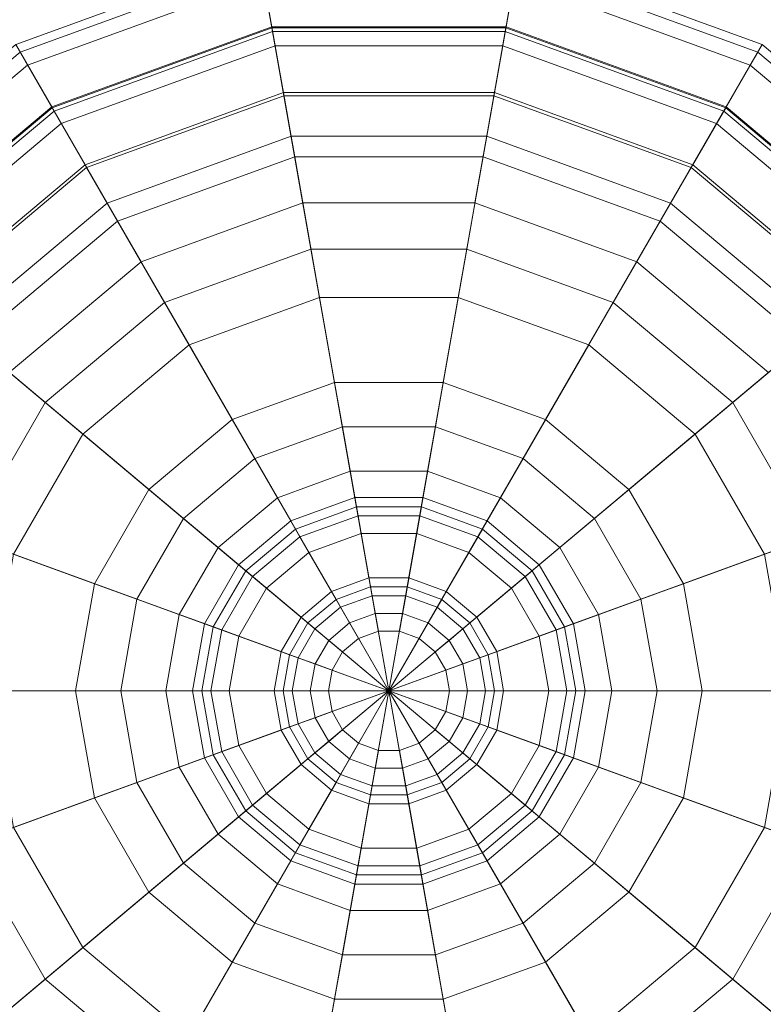
# Model space of a CAD drawing. Units: inches. Extents: x 375 to 1122, y 27 to 1069.
# Tile 99 of 155: x 718.593 to 719.942, y 864.699 to 866.486. Entities that reach past the tile are written whole.
import ezdxf

# ---------------------------------------------------------------- set-up
doc = ezdxf.new("R2010")
doc.units = ezdxf.units.IN
doc.layers.add('A-ANNO-DIMS', color=2, linetype='Continuous', lineweight=18)
doc.layers.add('Furniture', color=30, linetype='Continuous', lineweight=18)
doc.styles.get("Standard").update_dxf_attribs({"font": 'arial.ttf'})
doc.dimstyles.new('ISO-25', dxfattribs={"dimtxt": 12, "dimasz": 2.5, "dimexe": 1.5, "dimexo": 1.5, "dimtad": 1, "dimdec": 1, "dimlunit": 3, "dimtxsty": 'Standard', "dimblk": 'ARCHTICK', "dimcen": 2.5, "dimadec": 0, "dimazin": 0, "dimtfac": 1, "dimtdec": 1, "dimtmove": 0, "dimatfit": 3, "dimfxl": 1.5, "dimfxlon": 1, "dimarcsym": 0})

# ---------------------------------------------------------------- blocks, each defined once
blk = doc.blocks.new('A$C403C54AD')
for points in [[(1.826559, 0.891746, -0.031825), (1.826559, 0.857884, -0.028747), (1.826559, 0.857884, -0.028747), (1.814977, 0.889704, -0.031825)], [(1.83814, 0.889704, -0.031825), (1.826559, 0.857884, -0.028747), (1.826559, 0.857884, -0.028747), (1.826559, 0.891746, -0.031825)], [(1.814977, 0.889704, -0.031825), (1.826559, 0.857884, -0.028747), (1.826559, 0.857884, -0.028747), (1.804793, 0.883824, -0.031825)], [(1.848325, 0.883824, -0.031825), (1.826559, 0.857884, -0.028747), (1.826559, 0.857884, -0.028747), (1.83814, 0.889704, -0.031825)], [(1.826559, 0.872098, -0.02532), (1.826559, 0.88848, -0.028594), (1.816094, 0.886635, -0.028594), (1.821697, 0.871241, -0.02532)], [(1.83142, 0.871241, -0.02532), (1.837023, 0.886635, -0.028594), (1.826559, 0.88848, -0.028594), (1.826559, 0.872098, -0.02532)], [(1.821697, 0.871241, -0.02532), (1.816094, 0.886635, -0.028594), (1.806892, 0.881322, -0.028594), (1.817422, 0.868773, -0.02532)], [(1.835696, 0.868773, -0.02532), (1.846226, 0.881322, -0.028594), (1.837023, 0.886635, -0.028594), (1.83142, 0.871241, -0.02532)], [(1.806892, 0.881322, -0.028594), (1.804793, 0.883824, -0.031825), (1.797233, 0.874815, -0.031825), (1.800062, 0.873182, -0.028594)], [(1.804793, 0.883824, -0.031825), (1.826559, 0.857884, -0.028747), (1.826559, 0.857884, -0.028747), (1.797233, 0.874815, -0.031825)], [(1.855884, 0.874815, -0.031825), (1.826559, 0.857884, -0.028747), (1.826559, 0.857884, -0.028747), (1.848325, 0.883824, -0.031825)], [(1.806918, 0.881291, 0.131159), (1.805049, 0.883518, 0.117935), (1.797579, 0.874616, 0.117935), (1.800097, 0.873162, 0.131159)], [(1.805049, 0.883518, 0.117935), (1.805483, 0.883001, 0.089693), (1.798163, 0.874278, 0.089693), (1.797579, 0.874616, 0.117935)], [(1.817179, 0.883654, 0.071684), (1.819596, 0.877014, 0.061451), (1.813473, 0.873479, 0.061451), (1.808931, 0.878892, 0.071684)], [(1.844187, 0.878892, 0.071684), (1.839644, 0.873479, 0.061451), (1.833522, 0.877014, 0.061451), (1.835938, 0.883654, 0.071684)], [(1.805483, 0.883001, 0.089693), (1.808931, 0.878892, 0.071684), (1.802809, 0.871596, 0.071684), (1.798163, 0.874278, 0.089693)], [(1.817422, 0.868773, -0.02532), (1.806892, 0.881322, -0.028594), (1.800062, 0.873182, -0.028594), (1.814249, 0.864991, -0.02532)], [(1.81013, 0.877464, 0.140564), (1.806918, 0.881291, 0.131159), (1.800097, 0.873162, 0.131159), (1.804424, 0.870664, 0.140564)], [(1.807032, 0.881156, 0.117718), (1.808838, 0.879003, 0.130354), (1.802683, 0.871669, 0.130354), (1.80025, 0.873073, 0.117718)], [(1.807455, 0.880651, 0.090178), (1.807032, 0.881156, 0.117718), (1.80025, 0.873073, 0.117718), (1.80082, 0.872744, 0.090178)], [(1.838869, 0.864991, -0.02532), (1.853056, 0.873182, -0.028594), (1.846226, 0.881322, -0.028594), (1.835696, 0.868773, -0.02532)], [(1.820359, 0.874918, 0.063639), (1.818141, 0.881013, 0.073031), (1.810738, 0.876739, 0.073031), (1.814907, 0.87177, 0.063639)], [(1.838211, 0.87177, 0.063639), (1.84238, 0.876739, 0.073031), (1.834977, 0.881013, 0.073031), (1.832759, 0.874918, 0.063639)], [(1.810738, 0.876739, 0.073031), (1.807455, 0.880651, 0.090178), (1.80082, 0.872744, 0.090178), (1.805243, 0.87019, 0.073031)], [(1.808838, 0.879003, 0.130354), (1.812108, 0.875106, 0.140564), (1.80709, 0.869125, 0.140564), (1.802683, 0.871669, 0.130354)], [(1.808931, 0.878892, 0.071684), (1.813473, 0.873479, 0.061451), (1.808929, 0.868063, 0.061451), (1.802809, 0.871596, 0.071684)], [(1.850309, 0.871596, 0.071684), (1.844189, 0.868063, 0.061451), (1.839644, 0.873479, 0.061451), (1.844187, 0.878892, 0.071684)], [(1.826559, 0.878242, 0.061451), (1.826559, 0.868003, 0.054084), (1.823098, 0.867392, 0.054084), (1.819596, 0.877014, 0.061451)], [(1.833522, 0.877014, 0.061451), (1.83002, 0.867392, 0.054084), (1.826559, 0.868003, 0.054084), (1.826559, 0.878242, 0.061451)], [(1.812108, 0.875106, 0.140564), (1.81013, 0.877464, 0.140564), (1.804424, 0.870664, 0.140564), (1.80709, 0.869125, 0.140564)], [(1.814907, 0.87177, 0.063639), (1.810738, 0.876739, 0.073031), (1.805243, 0.87019, 0.073031), (1.81086, 0.866948, 0.063639)], [(1.819596, 0.877014, 0.061451), (1.823098, 0.867392, 0.054084), (1.820055, 0.865635, 0.054084), (1.813473, 0.873479, 0.061451)], [(1.839644, 0.873479, 0.061451), (1.833063, 0.865635, 0.054084), (1.83002, 0.867392, 0.054084), (1.833522, 0.877014, 0.061451)], [(1.842258, 0.866948, 0.063639), (1.847874, 0.87019, 0.073031), (1.84238, 0.876739, 0.073031), (1.838211, 0.87177, 0.063639)], [(1.826559, 0.866788, 0.057003), (1.826559, 0.876011, 0.063639), (1.820359, 0.874918, 0.063639), (1.823514, 0.866251, 0.057003)], [(1.829604, 0.866251, 0.057003), (1.832759, 0.874918, 0.063639), (1.826559, 0.876011, 0.063639), (1.826559, 0.866788, 0.057003)], [(1.823514, 0.866251, 0.057003), (1.820359, 0.874918, 0.063639), (1.814907, 0.87177, 0.063639), (1.820835, 0.864705, 0.057003)], [(1.832282, 0.864705, 0.057003), (1.838211, 0.87177, 0.063639), (1.832759, 0.874918, 0.063639), (1.829604, 0.866251, 0.057003)], [(1.800062, 0.873182, -0.028594), (1.797233, 0.874815, -0.031825), (1.793211, 0.863764, -0.031825), (1.796427, 0.863197, -0.028594)], [(1.797233, 0.874815, -0.031825), (1.826559, 0.857884, -0.028747), (1.826559, 0.857884, -0.028747), (1.793211, 0.863764, -0.031825)], [(1.800097, 0.873162, 0.131159), (1.797579, 0.874616, 0.117935), (1.793604, 0.863695, 0.117935), (1.796467, 0.86319, 0.131159)], [(1.797579, 0.874616, 0.117935), (1.798163, 0.874278, 0.089693), (1.794269, 0.863578, 0.089693), (1.793604, 0.863695, 0.117935)], [(1.859907, 0.863764, -0.031825), (1.826559, 0.857884, -0.028747), (1.826559, 0.857884, -0.028747), (1.855884, 0.874815, -0.031825)], [(1.798163, 0.874278, 0.089693), (1.802809, 0.871596, 0.071684), (1.799552, 0.862646, 0.071684), (1.794269, 0.863578, 0.089693)], [(1.814249, 0.864991, -0.02532), (1.800062, 0.873182, -0.028594), (1.796427, 0.863197, -0.028594), (1.812561, 0.860352, -0.02532)], [(1.804424, 0.870664, 0.140564), (1.800097, 0.873162, 0.131159), (1.796467, 0.86319, 0.131159), (1.801388, 0.862322, 0.140564)], [(1.813473, 0.873479, 0.061451), (1.820055, 0.865635, 0.054084), (1.817796, 0.862943, 0.054084), (1.808929, 0.868063, 0.061451)], [(1.844189, 0.868063, 0.061451), (1.835322, 0.862943, 0.054084), (1.833063, 0.865635, 0.054084), (1.839644, 0.873479, 0.061451)], [(1.840557, 0.860352, -0.02532), (1.85669, 0.863197, -0.028594), (1.853056, 0.873182, -0.028594), (1.838869, 0.864991, -0.02532)], [(1.80025, 0.873073, 0.117718), (1.802683, 0.871669, 0.130354), (1.799409, 0.862671, 0.130354), (1.796642, 0.863159, 0.117718)], [(1.80082, 0.872744, 0.090178), (1.80025, 0.873073, 0.117718), (1.796642, 0.863159, 0.117718), (1.79729, 0.863045, 0.090178)], [(1.805243, 0.87019, 0.073031), (1.80082, 0.872744, 0.090178), (1.79729, 0.863045, 0.090178), (1.80232, 0.862158, 0.073031)], [(1.820835, 0.864705, 0.057003), (1.814907, 0.87177, 0.063639), (1.81086, 0.866948, 0.063639), (1.818848, 0.862336, 0.057003)], [(1.826559, 0.87005, -0.022455), (1.826559, 0.872098, -0.02532), (1.821697, 0.871241, -0.02532), (1.822398, 0.869317, -0.022455)], [(1.83072, 0.869317, -0.022455), (1.83142, 0.871241, -0.02532), (1.826559, 0.872098, -0.02532), (1.826559, 0.87005, -0.022455)], [(1.83427, 0.862336, 0.057003), (1.842258, 0.866948, 0.063639), (1.838211, 0.87177, 0.063639), (1.832282, 0.864705, 0.057003)], [(1.802683, 0.871669, 0.130354), (1.80709, 0.869125, 0.140564), (1.804419, 0.861788, 0.140564), (1.799409, 0.862671, 0.130354)], [(1.802809, 0.871596, 0.071684), (1.808929, 0.868063, 0.061451), (1.806511, 0.861419, 0.061451), (1.799552, 0.862646, 0.071684)], [(1.822398, 0.869317, -0.022455), (1.821697, 0.871241, -0.02532), (1.817422, 0.868773, -0.02532), (1.818738, 0.867204, -0.022455)], [(1.834379, 0.867204, -0.022455), (1.835696, 0.868773, -0.02532), (1.83142, 0.871241, -0.02532), (1.83072, 0.869317, -0.022455)], [(1.80709, 0.869125, 0.140564), (1.804424, 0.870664, 0.140564), (1.801388, 0.862322, 0.140564), (1.804419, 0.861788, 0.140564)], [(1.81086, 0.866948, 0.063639), (1.805243, 0.87019, 0.073031), (1.80232, 0.862158, 0.073031), (1.808707, 0.861032, 0.063639)], [(1.826559, 0.865955, -0.020408), (1.826559, 0.87005, -0.022455), (1.822398, 0.869317, -0.022455), (1.823798, 0.865468, -0.020408)], [(1.829319, 0.865468, -0.020408), (1.83072, 0.869317, -0.022455), (1.826559, 0.87005, -0.022455), (1.826559, 0.865955, -0.020408)], [(1.823798, 0.865468, -0.020408), (1.822398, 0.869317, -0.022455), (1.818738, 0.867204, -0.022455), (1.821371, 0.864067, -0.020408)], [(1.831747, 0.864067, -0.020408), (1.834379, 0.867204, -0.022455), (1.83072, 0.869317, -0.022455), (1.829319, 0.865468, -0.020408)], [(1.818738, 0.867204, -0.022455), (1.817422, 0.868773, -0.02532), (1.814249, 0.864991, -0.02532), (1.816022, 0.863967, -0.022455)], [(1.837095, 0.863967, -0.022455), (1.838869, 0.864991, -0.02532), (1.835696, 0.868773, -0.02532), (1.834379, 0.867204, -0.022455)], [(1.808929, 0.868063, 0.061451), (1.817796, 0.862943, 0.054084), (1.816594, 0.859641, 0.054084), (1.806511, 0.861419, 0.061451)], [(1.826559, 0.868003, 0.054084), (1.826559, 0.863088, 0.053266), (1.824779, 0.862774, 0.053266), (1.823098, 0.867392, 0.054084)], [(1.83002, 0.867392, 0.054084), (1.828339, 0.862774, 0.053266), (1.826559, 0.863088, 0.053266), (1.826559, 0.868003, 0.054084)], [(1.846607, 0.861419, 0.061451), (1.836524, 0.859641, 0.054084), (1.835322, 0.862943, 0.054084), (1.844189, 0.868063, 0.061451)], [(1.823098, 0.867392, 0.054084), (1.824779, 0.862774, 0.053266), (1.823214, 0.861871, 0.053266), (1.820055, 0.865635, 0.054084)], [(1.833063, 0.865635, 0.054084), (1.829904, 0.861871, 0.053266), (1.828339, 0.862774, 0.053266), (1.83002, 0.867392, 0.054084)], [(1.818848, 0.862336, 0.057003), (1.81086, 0.866948, 0.063639), (1.808707, 0.861032, 0.063639), (1.81779, 0.85943, 0.057003)], [(1.821371, 0.864067, -0.020408), (1.818738, 0.867204, -0.022455), (1.816022, 0.863967, -0.022455), (1.819569, 0.861919, -0.020408)], [(1.833549, 0.861919, -0.020408), (1.837095, 0.863967, -0.022455), (1.834379, 0.867204, -0.022455), (1.831747, 0.864067, -0.020408)], [(1.835328, 0.85943, 0.057003), (1.844411, 0.861032, 0.063639), (1.842258, 0.866948, 0.063639), (1.83427, 0.862336, 0.057003)], [(1.826559, 0.857884, 0.055519), (1.826559, 0.866788, 0.057003), (1.823514, 0.866251, 0.057003), (1.826559, 0.857884, 0.055519)], [(1.826559, 0.857884, 0.055519), (1.829604, 0.866251, 0.057003), (1.826559, 0.866788, 0.057003), (1.826559, 0.857884, 0.055519)], [(1.826559, 0.857884, 0.055519), (1.823514, 0.866251, 0.057003), (1.820835, 0.864705, 0.057003), (1.826559, 0.857884, 0.055519)], [(1.826559, 0.866365, 0.0504), (1.826559, 0.862269, 0.048354), (1.825059, 0.862005, 0.048354), (1.823658, 0.865853, 0.0504)], [(1.826559, 0.865136, 0.052447), (1.826559, 0.866365, 0.0504), (1.823658, 0.865853, 0.0504), (1.824079, 0.864699, 0.052447)], [(1.826559, 0.862679, -0.015087), (1.826559, 0.865955, -0.020408), (1.823798, 0.865468, -0.020408), (1.824919, 0.862389, -0.015087)], [(1.829459, 0.865853, 0.0504), (1.828059, 0.862005, 0.048354), (1.826559, 0.862269, 0.048354), (1.826559, 0.866365, 0.0504)], [(1.829039, 0.864699, 0.052447), (1.829459, 0.865853, 0.0504), (1.826559, 0.866365, 0.0504), (1.826559, 0.865136, 0.052447)], [(1.826559, 0.857884, 0.055519), (1.832282, 0.864705, 0.057003), (1.829604, 0.866251, 0.057003), (1.826559, 0.857884, 0.055519)], [(1.828199, 0.862389, -0.015087), (1.829319, 0.865468, -0.020408), (1.826559, 0.865955, -0.020408), (1.826559, 0.862679, -0.015087)], [(1.820055, 0.865635, 0.054084), (1.823214, 0.861871, 0.053266), (1.822052, 0.860486, 0.053266), (1.817796, 0.862943, 0.054084)], [(1.823658, 0.865853, 0.0504), (1.825059, 0.862005, 0.048354), (1.82374, 0.861243, 0.048354), (1.821108, 0.86438, 0.0504)], [(1.824079, 0.864699, 0.052447), (1.823658, 0.865853, 0.0504), (1.821108, 0.86438, 0.0504), (1.821897, 0.863439, 0.052447)], [(1.83201, 0.86438, 0.0504), (1.829378, 0.861243, 0.048354), (1.828059, 0.862005, 0.048354), (1.829459, 0.865853, 0.0504)], [(1.83122, 0.863439, 0.052447), (1.83201, 0.86438, 0.0504), (1.829459, 0.865853, 0.0504), (1.829039, 0.864699, 0.052447)], [(1.835322, 0.862943, 0.054084), (1.831066, 0.860486, 0.053266), (1.829904, 0.861871, 0.053266), (1.833063, 0.865635, 0.054084)], [(1.824919, 0.862389, -0.015087), (1.823798, 0.865468, -0.020408), (1.821371, 0.864067, -0.020408), (1.823477, 0.861557, -0.015087)], [(1.826559, 0.863088, 0.053266), (1.826559, 0.865136, 0.052447), (1.824079, 0.864699, 0.052447), (1.824779, 0.862774, 0.053266)], [(1.828339, 0.862774, 0.053266), (1.829039, 0.864699, 0.052447), (1.826559, 0.865136, 0.052447), (1.826559, 0.863088, 0.053266)], [(1.829641, 0.861557, -0.015087), (1.831747, 0.864067, -0.020408), (1.829319, 0.865468, -0.020408), (1.828199, 0.862389, -0.015087)], [(1.816022, 0.863967, -0.022455), (1.814249, 0.864991, -0.02532), (1.812561, 0.860352, -0.02532), (1.814577, 0.859997, -0.022455)], [(1.826559, 0.857884, 0.055519), (1.820835, 0.864705, 0.057003), (1.818848, 0.862336, 0.057003), (1.826559, 0.857884, 0.055519)], [(1.824779, 0.862774, 0.053266), (1.824079, 0.864699, 0.052447), (1.821897, 0.863439, 0.052447), (1.823214, 0.861871, 0.053266)], [(1.826559, 0.857884, 0.055519), (1.83427, 0.862336, 0.057003), (1.832282, 0.864705, 0.057003), (1.826559, 0.857884, 0.055519)], [(1.829904, 0.861871, 0.053266), (1.83122, 0.863439, 0.052447), (1.829039, 0.864699, 0.052447), (1.828339, 0.862774, 0.053266)], [(1.838541, 0.859997, -0.022455), (1.840557, 0.860352, -0.02532), (1.838869, 0.864991, -0.02532), (1.837095, 0.863967, -0.022455)], [(1.821108, 0.86438, 0.0504), (1.82374, 0.861243, 0.048354), (1.822761, 0.860076, 0.048354), (1.819215, 0.862124, 0.0504)], [(1.821897, 0.863439, 0.052447), (1.821108, 0.86438, 0.0504), (1.819215, 0.862124, 0.0504), (1.820279, 0.86151, 0.052447)], [(1.833903, 0.862124, 0.0504), (1.830356, 0.860076, 0.048354), (1.829378, 0.861243, 0.048354), (1.83201, 0.86438, 0.0504)], [(1.832839, 0.86151, 0.052447), (1.833903, 0.862124, 0.0504), (1.83201, 0.86438, 0.0504), (1.83122, 0.863439, 0.052447)], [(1.796427, 0.863197, -0.028594), (1.793211, 0.863764, -0.031825), (1.793211, 0.852004, -0.031825), (1.796427, 0.852571, -0.028594)], [(1.793211, 0.863764, -0.031825), (1.826559, 0.857884, -0.028747), (1.826559, 0.857884, -0.028747), (1.793211, 0.852004, -0.031825)], [(1.819569, 0.861919, -0.020408), (1.816022, 0.863967, -0.022455), (1.814577, 0.859997, -0.022455), (1.818611, 0.859285, -0.020408)], [(1.823477, 0.861557, -0.015087), (1.821371, 0.864067, -0.020408), (1.819569, 0.861919, -0.020408), (1.822407, 0.860281, -0.015087)], [(1.859907, 0.852004, -0.031825), (1.826559, 0.857884, -0.028747), (1.826559, 0.857884, -0.028747), (1.859907, 0.863764, -0.031825)], [(1.830711, 0.860281, -0.015087), (1.833549, 0.861919, -0.020408), (1.831747, 0.864067, -0.020408), (1.829641, 0.861557, -0.015087)], [(1.834507, 0.859285, -0.020408), (1.838541, 0.859997, -0.022455), (1.837095, 0.863967, -0.022455), (1.833549, 0.861919, -0.020408)], [(1.796467, 0.86319, 0.131159), (1.793604, 0.863695, 0.117935), (1.793604, 0.852073, 0.117935), (1.796467, 0.852578, 0.131159)], [(1.794269, 0.863578, 0.089693), (1.799552, 0.862646, 0.071684), (1.799552, 0.853122, 0.071684), (1.794269, 0.85219, 0.089693)], [(1.823214, 0.861871, 0.053266), (1.821897, 0.863439, 0.052447), (1.820279, 0.86151, 0.052447), (1.822052, 0.860486, 0.053266)], [(1.831066, 0.860486, 0.053266), (1.832839, 0.86151, 0.052447), (1.83122, 0.863439, 0.052447), (1.829904, 0.861871, 0.053266)], [(1.812561, 0.860352, -0.02532), (1.796427, 0.863197, -0.028594), (1.796427, 0.852571, -0.028594), (1.812561, 0.855416, -0.02532)], [(1.801388, 0.862322, 0.140564), (1.796467, 0.86319, 0.131159), (1.796467, 0.852578, 0.131159), (1.801388, 0.853446, 0.140564)], [(1.796642, 0.863159, 0.117718), (1.799409, 0.862671, 0.130354), (1.799409, 0.853097, 0.130354), (1.796642, 0.852609, 0.117718)], [(1.79729, 0.863045, 0.090178), (1.796642, 0.863159, 0.117718), (1.796642, 0.852609, 0.117718), (1.79729, 0.852723, 0.090178)], [(1.80232, 0.862158, 0.073031), (1.79729, 0.863045, 0.090178), (1.79729, 0.852723, 0.090178), (1.80232, 0.85361, 0.073031)], [(1.817796, 0.862943, 0.054084), (1.822052, 0.860486, 0.053266), (1.821434, 0.858788, 0.053266), (1.816594, 0.859641, 0.054084)], [(1.836524, 0.859641, 0.054084), (1.831684, 0.858788, 0.053266), (1.831066, 0.860486, 0.053266), (1.835322, 0.862943, 0.054084)], [(1.840557, 0.855416, -0.02532), (1.85669, 0.852571, -0.028594), (1.85669, 0.863197, -0.028594), (1.840557, 0.860352, -0.02532)], [(1.799409, 0.862671, 0.130354), (1.804419, 0.861788, 0.140564), (1.804419, 0.85398, 0.140564), (1.799409, 0.853097, 0.130354)], [(1.799552, 0.862646, 0.071684), (1.806511, 0.861419, 0.061451), (1.806511, 0.854349, 0.061451), (1.799552, 0.853122, 0.071684)], [(1.825339, 0.861235, -0.006492), (1.824919, 0.862389, -0.015087), (1.823477, 0.861557, -0.015087), (1.824267, 0.860616, -0.006492)], [(1.826559, 0.86145, -0.006492), (1.826559, 0.862679, -0.015087), (1.824919, 0.862389, -0.015087), (1.825339, 0.861235, -0.006492)], [(1.827779, 0.861235, -0.006492), (1.828199, 0.862389, -0.015087), (1.826559, 0.862679, -0.015087), (1.826559, 0.86145, -0.006492)], [(1.828851, 0.860616, -0.006492), (1.829641, 0.861557, -0.015087), (1.828199, 0.862389, -0.015087), (1.827779, 0.861235, -0.006492)], [(1.804419, 0.861788, 0.140564), (1.801388, 0.862322, 0.140564), (1.801388, 0.853446, 0.140564), (1.804419, 0.85398, 0.140564)], [(1.808707, 0.861032, 0.063639), (1.80232, 0.862158, 0.073031), (1.80232, 0.85361, 0.073031), (1.808707, 0.854736, 0.063639)], [(1.826559, 0.857884, 0.055519), (1.818848, 0.862336, 0.057003), (1.81779, 0.85943, 0.057003), (1.826559, 0.857884, 0.055519)], [(1.820279, 0.86151, 0.052447), (1.819215, 0.862124, 0.0504), (1.818207, 0.859357, 0.0504), (1.819417, 0.859143, 0.052447)], [(1.819215, 0.862124, 0.0504), (1.822761, 0.860076, 0.048354), (1.82224, 0.858645, 0.048354), (1.818207, 0.859357, 0.0504)], [(1.822407, 0.860281, -0.015087), (1.819569, 0.861919, -0.020408), (1.818611, 0.859285, -0.020408), (1.821837, 0.858717, -0.015087)], [(1.825059, 0.862005, 0.048354), (1.825619, 0.860465, 0.041805), (1.824793, 0.859988, 0.041805), (1.82374, 0.861243, 0.048354)], [(1.826559, 0.862269, 0.048354), (1.826559, 0.860631, 0.041805), (1.825619, 0.860465, 0.041805), (1.825059, 0.862005, 0.048354)], [(1.826559, 0.857884, 0.055519), (1.835328, 0.85943, 0.057003), (1.83427, 0.862336, 0.057003), (1.826559, 0.857884, 0.055519)], [(1.828059, 0.862005, 0.048354), (1.827498, 0.860465, 0.041805), (1.826559, 0.860631, 0.041805), (1.826559, 0.862269, 0.048354)], [(1.829378, 0.861243, 0.048354), (1.828325, 0.859988, 0.041805), (1.827498, 0.860465, 0.041805), (1.828059, 0.862005, 0.048354)], [(1.834911, 0.859357, 0.0504), (1.830877, 0.858645, 0.048354), (1.830356, 0.860076, 0.048354), (1.833903, 0.862124, 0.0504)], [(1.831281, 0.858717, -0.015087), (1.834507, 0.859285, -0.020408), (1.833549, 0.861919, -0.020408), (1.830711, 0.860281, -0.015087)], [(1.833701, 0.859143, 0.052447), (1.834911, 0.859357, 0.0504), (1.833903, 0.862124, 0.0504), (1.832839, 0.86151, 0.052447)], [(1.822052, 0.860486, 0.053266), (1.820279, 0.86151, 0.052447), (1.819417, 0.859143, 0.052447), (1.821434, 0.858788, 0.053266)], [(1.824267, 0.860616, -0.006492), (1.823477, 0.861557, -0.015087), (1.822407, 0.860281, -0.015087), (1.823471, 0.859667, -0.006492)], [(1.829647, 0.859667, -0.006492), (1.830711, 0.860281, -0.015087), (1.829641, 0.861557, -0.015087), (1.828851, 0.860616, -0.006492)], [(1.831684, 0.858788, 0.053266), (1.833701, 0.859143, 0.052447), (1.832839, 0.86151, 0.052447), (1.831066, 0.860486, 0.053266)], [(1.806511, 0.861419, 0.061451), (1.816594, 0.859641, 0.054084), (1.816594, 0.856127, 0.054084), (1.806511, 0.854349, 0.061451)], [(1.81779, 0.85943, 0.057003), (1.808707, 0.861032, 0.063639), (1.808707, 0.854736, 0.063639), (1.81779, 0.856338, 0.057003)], [(1.82374, 0.861243, 0.048354), (1.824793, 0.859988, 0.041805), (1.82418, 0.859257, 0.041805), (1.822761, 0.860076, 0.048354)], [(1.825619, 0.860465, 0.041805), (1.825339, 0.861235, -0.006492), (1.824267, 0.860616, -0.006492), (1.824793, 0.859988, 0.041805)], [(1.826559, 0.860631, 0.041805), (1.826559, 0.86145, -0.006492), (1.825339, 0.861235, -0.006492), (1.825619, 0.860465, 0.041805)], [(1.827498, 0.860465, 0.041805), (1.827779, 0.861235, -0.006492), (1.826559, 0.86145, -0.006492), (1.826559, 0.860631, 0.041805)], [(1.828325, 0.859988, 0.041805), (1.828851, 0.860616, -0.006492), (1.827779, 0.861235, -0.006492), (1.827498, 0.860465, 0.041805)], [(1.830356, 0.860076, 0.048354), (1.828938, 0.859257, 0.041805), (1.828325, 0.859988, 0.041805), (1.829378, 0.861243, 0.048354)], [(1.835328, 0.856338, 0.057003), (1.844411, 0.854736, 0.063639), (1.844411, 0.861032, 0.063639), (1.835328, 0.85943, 0.057003)], [(1.846607, 0.854349, 0.061451), (1.836524, 0.856127, 0.054084), (1.836524, 0.859641, 0.054084), (1.846607, 0.861419, 0.061451)], [(1.824793, 0.859988, 0.041805), (1.824267, 0.860616, -0.006492), (1.823471, 0.859667, -0.006492), (1.82418, 0.859257, 0.041805)], [(1.828938, 0.859257, 0.041805), (1.829647, 0.859667, -0.006492), (1.828851, 0.860616, -0.006492), (1.828325, 0.859988, 0.041805)], [(1.814577, 0.859997, -0.022455), (1.812561, 0.860352, -0.02532), (1.812561, 0.855416, -0.02532), (1.814577, 0.855771, -0.022455)], [(1.823471, 0.859667, -0.006492), (1.822407, 0.860281, -0.015087), (1.821837, 0.858717, -0.015087), (1.823047, 0.858503, -0.006492)], [(1.830071, 0.858503, -0.006492), (1.831281, 0.858717, -0.015087), (1.830711, 0.860281, -0.015087), (1.829647, 0.859667, -0.006492)], [(1.838541, 0.855771, -0.022455), (1.840557, 0.855416, -0.02532), (1.840557, 0.860352, -0.02532), (1.838541, 0.859997, -0.022455)], [(1.818611, 0.859285, -0.020408), (1.814577, 0.859997, -0.022455), (1.814577, 0.855771, -0.022455), (1.818611, 0.856482, -0.020408)], [(1.822761, 0.860076, 0.048354), (1.82418, 0.859257, 0.041805), (1.823854, 0.858361, 0.041805), (1.82224, 0.858645, 0.048354)], [(1.830877, 0.858645, 0.048354), (1.829264, 0.858361, 0.041805), (1.828938, 0.859257, 0.041805), (1.830356, 0.860076, 0.048354)], [(1.834507, 0.856482, -0.020408), (1.838541, 0.855771, -0.022455), (1.838541, 0.859997, -0.022455), (1.834507, 0.859285, -0.020408)], [(1.816594, 0.859641, 0.054084), (1.821434, 0.858788, 0.053266), (1.821434, 0.85698, 0.053266), (1.816594, 0.856127, 0.054084)], [(1.826559, 0.857884, 0.055519), (1.81779, 0.85943, 0.057003), (1.81779, 0.856338, 0.057003), (1.826559, 0.857884, 0.055519)], [(1.819417, 0.859143, 0.052447), (1.818207, 0.859357, 0.0504), (1.818207, 0.856411, 0.0504), (1.819417, 0.856625, 0.052447)], [(1.818207, 0.859357, 0.0504), (1.82224, 0.858645, 0.048354), (1.82224, 0.857123, 0.048354), (1.818207, 0.856411, 0.0504)], [(1.821837, 0.858717, -0.015087), (1.818611, 0.859285, -0.020408), (1.818611, 0.856482, -0.020408), (1.821837, 0.857051, -0.015087)], [(1.82418, 0.859257, 0.041805), (1.823471, 0.859667, -0.006492), (1.823047, 0.858503, -0.006492), (1.823854, 0.858361, 0.041805)], [(1.826559, 0.857884, 0.055519), (1.835328, 0.856338, 0.057003), (1.835328, 0.85943, 0.057003), (1.826559, 0.857884, 0.055519)], [(1.829264, 0.858361, 0.041805), (1.830071, 0.858503, -0.006492), (1.829647, 0.859667, -0.006492), (1.828938, 0.859257, 0.041805)], [(1.834911, 0.856411, 0.0504), (1.830877, 0.857123, 0.048354), (1.830877, 0.858645, 0.048354), (1.834911, 0.859357, 0.0504)], [(1.831281, 0.857051, -0.015087), (1.834507, 0.856482, -0.020408), (1.834507, 0.859285, -0.020408), (1.831281, 0.858717, -0.015087)], [(1.836524, 0.856127, 0.054084), (1.831684, 0.85698, 0.053266), (1.831684, 0.858788, 0.053266), (1.836524, 0.859641, 0.054084)], [(1.833701, 0.856625, 0.052447), (1.834911, 0.856411, 0.0504), (1.834911, 0.859357, 0.0504), (1.833701, 0.859143, 0.052447)], [(1.821434, 0.858788, 0.053266), (1.819417, 0.859143, 0.052447), (1.819417, 0.856625, 0.052447), (1.821434, 0.85698, 0.053266)], [(1.831684, 0.85698, 0.053266), (1.833701, 0.856625, 0.052447), (1.833701, 0.859143, 0.052447), (1.831684, 0.858788, 0.053266)], [(1.823047, 0.858503, -0.006492), (1.821837, 0.858717, -0.015087), (1.821837, 0.857051, -0.015087), (1.823047, 0.857265, -0.006492)], [(1.82224, 0.858645, 0.048354), (1.823854, 0.858361, 0.041805), (1.823854, 0.857407, 0.041805), (1.82224, 0.857123, 0.048354)], [(1.823854, 0.858361, 0.041805), (1.823047, 0.858503, -0.006492), (1.823047, 0.857265, -0.006492), (1.823854, 0.857407, 0.041805)], [(1.830877, 0.857123, 0.048354), (1.829264, 0.857407, 0.041805), (1.829264, 0.858361, 0.041805), (1.830877, 0.858645, 0.048354)], [(1.829264, 0.857407, 0.041805), (1.830071, 0.857265, -0.006492), (1.830071, 0.858503, -0.006492), (1.829264, 0.858361, 0.041805)], [(1.830071, 0.857265, -0.006492), (1.831281, 0.857051, -0.015087), (1.831281, 0.858717, -0.015087), (1.830071, 0.858503, -0.006492)], [(1.793211, 0.852004, -0.031825), (1.826559, 0.857884, -0.028747), (1.826559, 0.857884, -0.028747), (1.797233, 0.840953, -0.031825)], [(1.797233, 0.840953, -0.031825), (1.826559, 0.857884, -0.028747), (1.826559, 0.857884, -0.028747), (1.804793, 0.831944, -0.031825)], [(1.804793, 0.831944, -0.031825), (1.826559, 0.857884, -0.028747), (1.826559, 0.857884, -0.028747), (1.814977, 0.826064, -0.031825)], [(1.814977, 0.826064, -0.031825), (1.826559, 0.857884, -0.028747), (1.826559, 0.857884, -0.028747), (1.826559, 0.824022, -0.031825)], [(1.826559, 0.857884, 0.055519), (1.81779, 0.856338, 0.057003), (1.818848, 0.853432, 0.057003), (1.826559, 0.857884, 0.055519)], [(1.826559, 0.857884, 0.055519), (1.818848, 0.853432, 0.057003), (1.820835, 0.851063, 0.057003), (1.826559, 0.857884, 0.055519)], [(1.826559, 0.857884, 0.055519), (1.820835, 0.851063, 0.057003), (1.823514, 0.849517, 0.057003), (1.826559, 0.857884, 0.055519)], [(1.826559, 0.857884, 0.055519), (1.823514, 0.849517, 0.057003), (1.826559, 0.84898, 0.057003), (1.826559, 0.857884, 0.055519)], [(1.826559, 0.857884, 0.055519), (1.83427, 0.853432, 0.057003), (1.835328, 0.856338, 0.057003), (1.826559, 0.857884, 0.055519)], [(1.826559, 0.857884, 0.055519), (1.832282, 0.851063, 0.057003), (1.83427, 0.853432, 0.057003), (1.826559, 0.857884, 0.055519)], [(1.826559, 0.857884, 0.055519), (1.829604, 0.849517, 0.057003), (1.832282, 0.851063, 0.057003), (1.826559, 0.857884, 0.055519)], [(1.826559, 0.857884, 0.055519), (1.826559, 0.84898, 0.057003), (1.829604, 0.849517, 0.057003), (1.826559, 0.857884, 0.055519)], [(1.855884, 0.840953, -0.031825), (1.826559, 0.857884, -0.028747), (1.826559, 0.857884, -0.028747), (1.859907, 0.852004, -0.031825)], [(1.848325, 0.831944, -0.031825), (1.826559, 0.857884, -0.028747), (1.826559, 0.857884, -0.028747), (1.855884, 0.840953, -0.031825)], [(1.83814, 0.826064, -0.031825), (1.826559, 0.857884, -0.028747), (1.826559, 0.857884, -0.028747), (1.848325, 0.831944, -0.031825)], [(1.826559, 0.824022, -0.031825), (1.826559, 0.857884, -0.028747), (1.826559, 0.857884, -0.028747), (1.83814, 0.826064, -0.031825)], [(1.818207, 0.856411, 0.0504), (1.82224, 0.857123, 0.048354), (1.822761, 0.855691, 0.048354), (1.819215, 0.853644, 0.0504)], [(1.821837, 0.857051, -0.015087), (1.818611, 0.856482, -0.020408), (1.819569, 0.853848, -0.020408), (1.822407, 0.855487, -0.015087)], [(1.823047, 0.857265, -0.006492), (1.821837, 0.857051, -0.015087), (1.822407, 0.855487, -0.015087), (1.823471, 0.856101, -0.006492)], [(1.82224, 0.857123, 0.048354), (1.823854, 0.857407, 0.041805), (1.82418, 0.856511, 0.041805), (1.822761, 0.855691, 0.048354)], [(1.823854, 0.857407, 0.041805), (1.823047, 0.857265, -0.006492), (1.823471, 0.856101, -0.006492), (1.82418, 0.856511, 0.041805)], [(1.830356, 0.855691, 0.048354), (1.828938, 0.856511, 0.041805), (1.829264, 0.857407, 0.041805), (1.830877, 0.857123, 0.048354)], [(1.828938, 0.856511, 0.041805), (1.829647, 0.856101, -0.006492), (1.830071, 0.857265, -0.006492), (1.829264, 0.857407, 0.041805)], [(1.829647, 0.856101, -0.006492), (1.830711, 0.855487, -0.015087), (1.831281, 0.857051, -0.015087), (1.830071, 0.857265, -0.006492)], [(1.833903, 0.853644, 0.0504), (1.830356, 0.855691, 0.048354), (1.830877, 0.857123, 0.048354), (1.834911, 0.856411, 0.0504)], [(1.830711, 0.855487, -0.015087), (1.833549, 0.853848, -0.020408), (1.834507, 0.856482, -0.020408), (1.831281, 0.857051, -0.015087)], [(1.816594, 0.856127, 0.054084), (1.821434, 0.85698, 0.053266), (1.822052, 0.855282, 0.053266), (1.817796, 0.852825, 0.054084)], [(1.819417, 0.856625, 0.052447), (1.818207, 0.856411, 0.0504), (1.819215, 0.853644, 0.0504), (1.820279, 0.854258, 0.052447)], [(1.821434, 0.85698, 0.053266), (1.819417, 0.856625, 0.052447), (1.820279, 0.854258, 0.052447), (1.822052, 0.855282, 0.053266)], [(1.831066, 0.855282, 0.053266), (1.832839, 0.854258, 0.052447), (1.833701, 0.856625, 0.052447), (1.831684, 0.85698, 0.053266)], [(1.835322, 0.852825, 0.054084), (1.831066, 0.855282, 0.053266), (1.831684, 0.85698, 0.053266), (1.836524, 0.856127, 0.054084)], [(1.832839, 0.854258, 0.052447), (1.833903, 0.853644, 0.0504), (1.834911, 0.856411, 0.0504), (1.833701, 0.856625, 0.052447)], [(1.806511, 0.854349, 0.061451), (1.816594, 0.856127, 0.054084), (1.817796, 0.852825, 0.054084), (1.808929, 0.847705, 0.061451)], [(1.81779, 0.856338, 0.057003), (1.808707, 0.854736, 0.063639), (1.81086, 0.84882, 0.063639), (1.818848, 0.853432, 0.057003)], [(1.818611, 0.856482, -0.020408), (1.814577, 0.855771, -0.022455), (1.816022, 0.851801, -0.022455), (1.819569, 0.853848, -0.020408)], [(1.822761, 0.855691, 0.048354), (1.82418, 0.856511, 0.041805), (1.824793, 0.85578, 0.041805), (1.82374, 0.854525, 0.048354)], [(1.82418, 0.856511, 0.041805), (1.823471, 0.856101, -0.006492), (1.824267, 0.855152, -0.006492), (1.824793, 0.85578, 0.041805)], [(1.829378, 0.854525, 0.048354), (1.828325, 0.85578, 0.041805), (1.828938, 0.856511, 0.041805), (1.830356, 0.855691, 0.048354)], [(1.828325, 0.85578, 0.041805), (1.828851, 0.855152, -0.006492), (1.829647, 0.856101, -0.006492), (1.828938, 0.856511, 0.041805)], [(1.833549, 0.853848, -0.020408), (1.837095, 0.851801, -0.022455), (1.838541, 0.855771, -0.022455), (1.834507, 0.856482, -0.020408)], [(1.83427, 0.853432, 0.057003), (1.842258, 0.84882, 0.063639), (1.844411, 0.854736, 0.063639), (1.835328, 0.856338, 0.057003)], [(1.844189, 0.847705, 0.061451), (1.835322, 0.852825, 0.054084), (1.836524, 0.856127, 0.054084), (1.846607, 0.854349, 0.061451)], [(1.814577, 0.855771, -0.022455), (1.812561, 0.855416, -0.02532), (1.814249, 0.850777, -0.02532), (1.816022, 0.851801, -0.022455)], [(1.819215, 0.853644, 0.0504), (1.822761, 0.855691, 0.048354), (1.82374, 0.854525, 0.048354), (1.821108, 0.851387, 0.0504)], [(1.823471, 0.856101, -0.006492), (1.822407, 0.855487, -0.015087), (1.823477, 0.854211, -0.015087), (1.824267, 0.855152, -0.006492)], [(1.82374, 0.854525, 0.048354), (1.824793, 0.85578, 0.041805), (1.825619, 0.855303, 0.041805), (1.825059, 0.853763, 0.048354)], [(1.824793, 0.85578, 0.041805), (1.824267, 0.855152, -0.006492), (1.825339, 0.854533, -0.006492), (1.825619, 0.855303, 0.041805)], [(1.828059, 0.853763, 0.048354), (1.827498, 0.855303, 0.041805), (1.828325, 0.85578, 0.041805), (1.829378, 0.854525, 0.048354)], [(1.827498, 0.855303, 0.041805), (1.827779, 0.854533, -0.006492), (1.828851, 0.855152, -0.006492), (1.828325, 0.85578, 0.041805)], [(1.828851, 0.855152, -0.006492), (1.829641, 0.854211, -0.015087), (1.830711, 0.855487, -0.015087), (1.829647, 0.856101, -0.006492)], [(1.83201, 0.851387, 0.0504), (1.829378, 0.854525, 0.048354), (1.830356, 0.855691, 0.048354), (1.833903, 0.853644, 0.0504)], [(1.837095, 0.851801, -0.022455), (1.838869, 0.850777, -0.02532), (1.840557, 0.855416, -0.02532), (1.838541, 0.855771, -0.022455)], [(1.812561, 0.855416, -0.02532), (1.796427, 0.852571, -0.028594), (1.800062, 0.842586, -0.028594), (1.814249, 0.850777, -0.02532)], [(1.817796, 0.852825, 0.054084), (1.822052, 0.855282, 0.053266), (1.823214, 0.853897, 0.053266), (1.820055, 0.850133, 0.054084)], [(1.822407, 0.855487, -0.015087), (1.819569, 0.853848, -0.020408), (1.821371, 0.851701, -0.020408), (1.823477, 0.854211, -0.015087)], [(1.822052, 0.855282, 0.053266), (1.820279, 0.854258, 0.052447), (1.821897, 0.852329, 0.052447), (1.823214, 0.853897, 0.053266)], [(1.825059, 0.853763, 0.048354), (1.825619, 0.855303, 0.041805), (1.826559, 0.855137, 0.041805), (1.826559, 0.853499, 0.048354)], [(1.825619, 0.855303, 0.041805), (1.825339, 0.854533, -0.006492), (1.826559, 0.854318, -0.006492), (1.826559, 0.855137, 0.041805)], [(1.826559, 0.853499, 0.048354), (1.826559, 0.855137, 0.041805), (1.827498, 0.855303, 0.041805), (1.828059, 0.853763, 0.048354)], [(1.826559, 0.855137, 0.041805), (1.826559, 0.854318, -0.006492), (1.827779, 0.854533, -0.006492), (1.827498, 0.855303, 0.041805)], [(1.829641, 0.854211, -0.015087), (1.831747, 0.851701, -0.020408), (1.833549, 0.853848, -0.020408), (1.830711, 0.855487, -0.015087)], [(1.829904, 0.853897, 0.053266), (1.83122, 0.852329, 0.052447), (1.832839, 0.854258, 0.052447), (1.831066, 0.855282, 0.053266)], [(1.833063, 0.850133, 0.054084), (1.829904, 0.853897, 0.053266), (1.831066, 0.855282, 0.053266), (1.835322, 0.852825, 0.054084)], [(1.838869, 0.850777, -0.02532), (1.853056, 0.842586, -0.028594), (1.85669, 0.852571, -0.028594), (1.840557, 0.855416, -0.02532)], [(1.824267, 0.855152, -0.006492), (1.823477, 0.854211, -0.015087), (1.824919, 0.853379, -0.015087), (1.825339, 0.854533, -0.006492)], [(1.827779, 0.854533, -0.006492), (1.828199, 0.853379, -0.015087), (1.829641, 0.854211, -0.015087), (1.828851, 0.855152, -0.006492)], [(1.799552, 0.853122, 0.071684), (1.806511, 0.854349, 0.061451), (1.808929, 0.847705, 0.061451), (1.802809, 0.844172, 0.071684)], [(1.808707, 0.854736, 0.063639), (1.80232, 0.85361, 0.073031), (1.805243, 0.845577, 0.073031), (1.81086, 0.84882, 0.063639)], [(1.821108, 0.851387, 0.0504), (1.82374, 0.854525, 0.048354), (1.825059, 0.853763, 0.048354), (1.823658, 0.849915, 0.0504)], [(1.825339, 0.854533, -0.006492), (1.824919, 0.853379, -0.015087), (1.826559, 0.853089, -0.015087), (1.826559, 0.854318, -0.006492)], [(1.826559, 0.854318, -0.006492), (1.826559, 0.853089, -0.015087), (1.828199, 0.853379, -0.015087), (1.827779, 0.854533, -0.006492)], [(1.829459, 0.849915, 0.0504), (1.828059, 0.853763, 0.048354), (1.829378, 0.854525, 0.048354), (1.83201, 0.851387, 0.0504)], [(1.799409, 0.853097, 0.130354), (1.804419, 0.85398, 0.140564), (1.80709, 0.846643, 0.140564), (1.802683, 0.844099, 0.130354)], [(1.804419, 0.85398, 0.140564), (1.801388, 0.853446, 0.140564), (1.804424, 0.845104, 0.140564), (1.80709, 0.846643, 0.140564)], [(1.820279, 0.854258, 0.052447), (1.819215, 0.853644, 0.0504), (1.821108, 0.851387, 0.0504), (1.821897, 0.852329, 0.052447)], [(1.820055, 0.850133, 0.054084), (1.823214, 0.853897, 0.053266), (1.824779, 0.852994, 0.053266), (1.823098, 0.848375, 0.054084)], [(1.823477, 0.854211, -0.015087), (1.821371, 0.851701, -0.020408), (1.823798, 0.8503, -0.020408), (1.824919, 0.853379, -0.015087)], [(1.823214, 0.853897, 0.053266), (1.821897, 0.852329, 0.052447), (1.824079, 0.851069, 0.052447), (1.824779, 0.852994, 0.053266)], [(1.828199, 0.853379, -0.015087), (1.829319, 0.8503, -0.020408), (1.831747, 0.851701, -0.020408), (1.829641, 0.854211, -0.015087)], [(1.828339, 0.852994, 0.053266), (1.829039, 0.851069, 0.052447), (1.83122, 0.852329, 0.052447), (1.829904, 0.853897, 0.053266)], [(1.83002, 0.848375, 0.054084), (1.828339, 0.852994, 0.053266), (1.829904, 0.853897, 0.053266), (1.833063, 0.850133, 0.054084)], [(1.83122, 0.852329, 0.052447), (1.83201, 0.851387, 0.0504), (1.833903, 0.853644, 0.0504), (1.832839, 0.854258, 0.052447)], [(1.801388, 0.853446, 0.140564), (1.796467, 0.852578, 0.131159), (1.800097, 0.842606, 0.131159), (1.804424, 0.845104, 0.140564)], [(1.80232, 0.85361, 0.073031), (1.79729, 0.852723, 0.090178), (1.80082, 0.843024, 0.090178), (1.805243, 0.845577, 0.073031)], [(1.818848, 0.853432, 0.057003), (1.81086, 0.84882, 0.063639), (1.814907, 0.843998, 0.063639), (1.820835, 0.851063, 0.057003)], [(1.819569, 0.853848, -0.020408), (1.816022, 0.851801, -0.022455), (1.818738, 0.848564, -0.022455), (1.821371, 0.851701, -0.020408)], [(1.823658, 0.849915, 0.0504), (1.825059, 0.853763, 0.048354), (1.826559, 0.853499, 0.048354), (1.826559, 0.849403, 0.0504)], [(1.826559, 0.849403, 0.0504), (1.826559, 0.853499, 0.048354), (1.828059, 0.853763, 0.048354), (1.829459, 0.849915, 0.0504)], [(1.831747, 0.851701, -0.020408), (1.834379, 0.848564, -0.022455), (1.837095, 0.851801, -0.022455), (1.833549, 0.853848, -0.020408)], [(1.832282, 0.851063, 0.057003), (1.838211, 0.843998, 0.063639), (1.842258, 0.84882, 0.063639), (1.83427, 0.853432, 0.057003)], [(1.794269, 0.85219, 0.089693), (1.799552, 0.853122, 0.071684), (1.802809, 0.844172, 0.071684), (1.798163, 0.84149, 0.089693)], [(1.796642, 0.852609, 0.117718), (1.799409, 0.853097, 0.130354), (1.802683, 0.844099, 0.130354), (1.80025, 0.842695, 0.117718)], [(1.823098, 0.848375, 0.054084), (1.824779, 0.852994, 0.053266), (1.826559, 0.85268, 0.053266), (1.826559, 0.847765, 0.054084)], [(1.824919, 0.853379, -0.015087), (1.823798, 0.8503, -0.020408), (1.826559, 0.849813, -0.020408), (1.826559, 0.853089, -0.015087)], [(1.824779, 0.852994, 0.053266), (1.824079, 0.851069, 0.052447), (1.826559, 0.850632, 0.052447), (1.826559, 0.85268, 0.053266)], [(1.826559, 0.853089, -0.015087), (1.826559, 0.849813, -0.020408), (1.829319, 0.8503, -0.020408), (1.828199, 0.853379, -0.015087)], [(1.826559, 0.85268, 0.053266), (1.826559, 0.850632, 0.052447), (1.829039, 0.851069, 0.052447), (1.828339, 0.852994, 0.053266)], [(1.826559, 0.847765, 0.054084), (1.826559, 0.85268, 0.053266), (1.828339, 0.852994, 0.053266), (1.83002, 0.848375, 0.054084)], [(1.796427, 0.852571, -0.028594), (1.793211, 0.852004, -0.031825), (1.797233, 0.840953, -0.031825), (1.800062, 0.842586, -0.028594)], [(1.796467, 0.852578, 0.131159), (1.793604, 0.852073, 0.117935), (1.797579, 0.841152, 0.117935), (1.800097, 0.842606, 0.131159)], [(1.79729, 0.852723, 0.090178), (1.796642, 0.852609, 0.117718), (1.80025, 0.842695, 0.117718), (1.80082, 0.843024, 0.090178)], [(1.808929, 0.847705, 0.061451), (1.817796, 0.852825, 0.054084), (1.820055, 0.850133, 0.054084), (1.813473, 0.842289, 0.061451)], [(1.839644, 0.842289, 0.061451), (1.833063, 0.850133, 0.054084), (1.835322, 0.852825, 0.054084), (1.844189, 0.847705, 0.061451)], [(1.793604, 0.852073, 0.117935), (1.794269, 0.85219, 0.089693), (1.798163, 0.84149, 0.089693), (1.797579, 0.841152, 0.117935)], [(1.821897, 0.852329, 0.052447), (1.821108, 0.851387, 0.0504), (1.823658, 0.849915, 0.0504), (1.824079, 0.851069, 0.052447)], [(1.829039, 0.851069, 0.052447), (1.829459, 0.849915, 0.0504), (1.83201, 0.851387, 0.0504), (1.83122, 0.852329, 0.052447)], [(1.816022, 0.851801, -0.022455), (1.814249, 0.850777, -0.02532), (1.817422, 0.846995, -0.02532), (1.818738, 0.848564, -0.022455)], [(1.821371, 0.851701, -0.020408), (1.818738, 0.848564, -0.022455), (1.822398, 0.846451, -0.022455), (1.823798, 0.8503, -0.020408)], [(1.829319, 0.8503, -0.020408), (1.83072, 0.846451, -0.022455), (1.834379, 0.848564, -0.022455), (1.831747, 0.851701, -0.020408)], [(1.834379, 0.848564, -0.022455), (1.835696, 0.846995, -0.02532), (1.838869, 0.850777, -0.02532), (1.837095, 0.851801, -0.022455)], [(1.814249, 0.850777, -0.02532), (1.800062, 0.842586, -0.028594), (1.806892, 0.834446, -0.028594), (1.817422, 0.846995, -0.02532)], [(1.820835, 0.851063, 0.057003), (1.814907, 0.843998, 0.063639), (1.820359, 0.84085, 0.063639), (1.823514, 0.849517, 0.057003)], [(1.824079, 0.851069, 0.052447), (1.823658, 0.849915, 0.0504), (1.826559, 0.849403, 0.0504), (1.826559, 0.850632, 0.052447)], [(1.826559, 0.850632, 0.052447), (1.826559, 0.849403, 0.0504), (1.829459, 0.849915, 0.0504), (1.829039, 0.851069, 0.052447)], [(1.829604, 0.849517, 0.057003), (1.832759, 0.84085, 0.063639), (1.838211, 0.843998, 0.063639), (1.832282, 0.851063, 0.057003)], [(1.835696, 0.846995, -0.02532), (1.846226, 0.834446, -0.028594), (1.853056, 0.842586, -0.028594), (1.838869, 0.850777, -0.02532)], [(1.813473, 0.842289, 0.061451), (1.820055, 0.850133, 0.054084), (1.823098, 0.848375, 0.054084), (1.819596, 0.838754, 0.061451)], [(1.823798, 0.8503, -0.020408), (1.822398, 0.846451, -0.022455), (1.826559, 0.845717, -0.022455), (1.826559, 0.849813, -0.020408)], [(1.826559, 0.849813, -0.020408), (1.826559, 0.845717, -0.022455), (1.83072, 0.846451, -0.022455), (1.829319, 0.8503, -0.020408)], [(1.833522, 0.838754, 0.061451), (1.83002, 0.848375, 0.054084), (1.833063, 0.850133, 0.054084), (1.839644, 0.842289, 0.061451)], [(1.823514, 0.849517, 0.057003), (1.820359, 0.84085, 0.063639), (1.826559, 0.839757, 0.063639), (1.826559, 0.84898, 0.057003)], [(1.826559, 0.84898, 0.057003), (1.826559, 0.839757, 0.063639), (1.832759, 0.84085, 0.063639), (1.829604, 0.849517, 0.057003)], [(1.81086, 0.84882, 0.063639), (1.805243, 0.845577, 0.073031), (1.810738, 0.839029, 0.073031), (1.814907, 0.843998, 0.063639)], [(1.818738, 0.848564, -0.022455), (1.817422, 0.846995, -0.02532), (1.821697, 0.844527, -0.02532), (1.822398, 0.846451, -0.022455)], [(1.83072, 0.846451, -0.022455), (1.83142, 0.844527, -0.02532), (1.835696, 0.846995, -0.02532), (1.834379, 0.848564, -0.022455)], [(1.838211, 0.843998, 0.063639), (1.84238, 0.839029, 0.073031), (1.847874, 0.845577, 0.073031), (1.842258, 0.84882, 0.063639)], [(1.819596, 0.838754, 0.061451), (1.823098, 0.848375, 0.054084), (1.826559, 0.847765, 0.054084), (1.826559, 0.837526, 0.061451)], [(1.826559, 0.837526, 0.061451), (1.826559, 0.847765, 0.054084), (1.83002, 0.848375, 0.054084), (1.833522, 0.838754, 0.061451)], [(1.802809, 0.844172, 0.071684), (1.808929, 0.847705, 0.061451), (1.813473, 0.842289, 0.061451), (1.808931, 0.836876, 0.071684)], [(1.844187, 0.836876, 0.071684), (1.839644, 0.842289, 0.061451), (1.844189, 0.847705, 0.061451), (1.850309, 0.844172, 0.071684)], [(1.817422, 0.846995, -0.02532), (1.806892, 0.834446, -0.028594), (1.816094, 0.829133, -0.028594), (1.821697, 0.844527, -0.02532)], [(1.83142, 0.844527, -0.02532), (1.837023, 0.829133, -0.028594), (1.846226, 0.834446, -0.028594), (1.835696, 0.846995, -0.02532)], [(1.802683, 0.844099, 0.130354), (1.80709, 0.846643, 0.140564), (1.812108, 0.840662, 0.140564), (1.808838, 0.836765, 0.130354)], [(1.80709, 0.846643, 0.140564), (1.804424, 0.845104, 0.140564), (1.81013, 0.838304, 0.140564), (1.812108, 0.840662, 0.140564)], [(1.822398, 0.846451, -0.022455), (1.821697, 0.844527, -0.02532), (1.826559, 0.84367, -0.02532), (1.826559, 0.845717, -0.022455)], [(1.826559, 0.845717, -0.022455), (1.826559, 0.84367, -0.02532), (1.83142, 0.844527, -0.02532), (1.83072, 0.846451, -0.022455)], [(1.805243, 0.845577, 0.073031), (1.80082, 0.843024, 0.090178), (1.807455, 0.835117, 0.090178), (1.810738, 0.839029, 0.073031)], [(1.804424, 0.845104, 0.140564), (1.800097, 0.842606, 0.131159), (1.806918, 0.834477, 0.131159), (1.81013, 0.838304, 0.140564)], [(1.821697, 0.844527, -0.02532), (1.816094, 0.829133, -0.028594), (1.826559, 0.827288, -0.028594), (1.826559, 0.84367, -0.02532)], [(1.826559, 0.84367, -0.02532), (1.826559, 0.827288, -0.028594), (1.837023, 0.829133, -0.028594), (1.83142, 0.844527, -0.02532)], [(1.798163, 0.84149, 0.089693), (1.802809, 0.844172, 0.071684), (1.808931, 0.836876, 0.071684), (1.805483, 0.832767, 0.089693)], [(1.80025, 0.842695, 0.117718), (1.802683, 0.844099, 0.130354), (1.808838, 0.836765, 0.130354), (1.807032, 0.834612, 0.117718)], [(1.814907, 0.843998, 0.063639), (1.810738, 0.839029, 0.073031), (1.818141, 0.834755, 0.073031), (1.820359, 0.84085, 0.063639)], [(1.832759, 0.84085, 0.063639), (1.834977, 0.834755, 0.073031), (1.84238, 0.839029, 0.073031), (1.838211, 0.843998, 0.063639)], [(1.80082, 0.843024, 0.090178), (1.80025, 0.842695, 0.117718), (1.807032, 0.834612, 0.117718), (1.807455, 0.835117, 0.090178)], [(1.800062, 0.842586, -0.028594), (1.797233, 0.840953, -0.031825), (1.804793, 0.831944, -0.031825), (1.806892, 0.834446, -0.028594)], [(1.800097, 0.842606, 0.131159), (1.797579, 0.841152, 0.117935), (1.805049, 0.83225, 0.117935), (1.806918, 0.834477, 0.131159)], [(1.808931, 0.836876, 0.071684), (1.813473, 0.842289, 0.061451), (1.819596, 0.838754, 0.061451), (1.817179, 0.832114, 0.071684)], [(1.835938, 0.832114, 0.071684), (1.833522, 0.838754, 0.061451), (1.839644, 0.842289, 0.061451), (1.844187, 0.836876, 0.071684)], [(1.797579, 0.841152, 0.117935), (1.798163, 0.84149, 0.089693), (1.805483, 0.832767, 0.089693), (1.805049, 0.83225, 0.117935)]]:
    blk.add_3dface(points)
blk = doc.blocks.new('_ArchTick')
at = {"color": 0, "linetype": 'ByBlock', "const_width": 0.15}
blk.add_lwpolyline([(-0.5, -0.5), (0.5, 0.5)], dxfattribs=at)
blk = doc.blocks.new('*D85')
at = {"layer": 'A-ANNO-DIMS', "color": 0, "lineweight": -2, "transparency": 16777216}
for p, q in [((401.5073, 868.5277), (398.5073, 868.5277)), ((400.0073, 814.5277), (400.0073, 868.5277)), ((401.5073, 814.5277), (398.5073, 814.5277))]:
    blk.add_line(p, q, dxfattribs=at)
at = {"layer": 'Defpoints', "color": 0, "transparency": 16777216}
for p in [(400.0073, 868.5277), (845.0073, 868.5277), (845.0073, 814.5277)]:
    blk.add_point(p, dxfattribs=at)
at = {"layer": 'A-ANNO-DIMS', "color": 0, "lineweight": -2, "transparency": 16777216, "xscale": 2.5, "yscale": 2.5, "zscale": 2.5}
for p, rotation in [((400.0073, 868.5277), 90), ((400.0073, 814.5277), 270)]:
    blk.add_blockref('_ArchTick', p, dxfattribs=dict(at, rotation=rotation))
at = {"layer": 'A-ANNO-DIMS', "color": 0, "transparency": 16777216, "insert": (393.2555, 841.5277), "char_height": 12, "attachment_point": 5, "rotation": 90}
blk.add_mtext('4\'-6"', dxfattribs=at)

msp = doc.modelspace()

# ---------------------------------------------------------------- block references
at = {"layer": 'Furniture', "xscale": 39.9918517141215, "yscale": 39.9918517141215, "zscale": 39.9918517141215, "rotation": 270}
msp.add_blockref('A$C403C54AD', (684.9549, 938.3156, 0.024), dxfattribs=at)

# ---------------------------------------------------------------- dimensions: what is measured, and where the dimension line sits
at = {"layer": 'A-ANNO-DIMS'}
dim = msp.add_linear_dim(base=(400.0073, 868.5277), p1=(845.0073, 814.5277), p2=(845.0073, 868.5277), angle=90, dimstyle='ISO-25', override={"dimdec": 1, "dimlfac": 1, "dimrnd": 0, "dimzin": 1, "dimdsep": 46, "dimlunit": 4, "dimfrac": 2}, dxfattribs=at)
dim.commit()
dim.dimension.update_dxf_attribs({"geometry": '*D85', "text_midpoint": (393.2555, 841.5277)})

doc.saveas('drawing.dxf')
